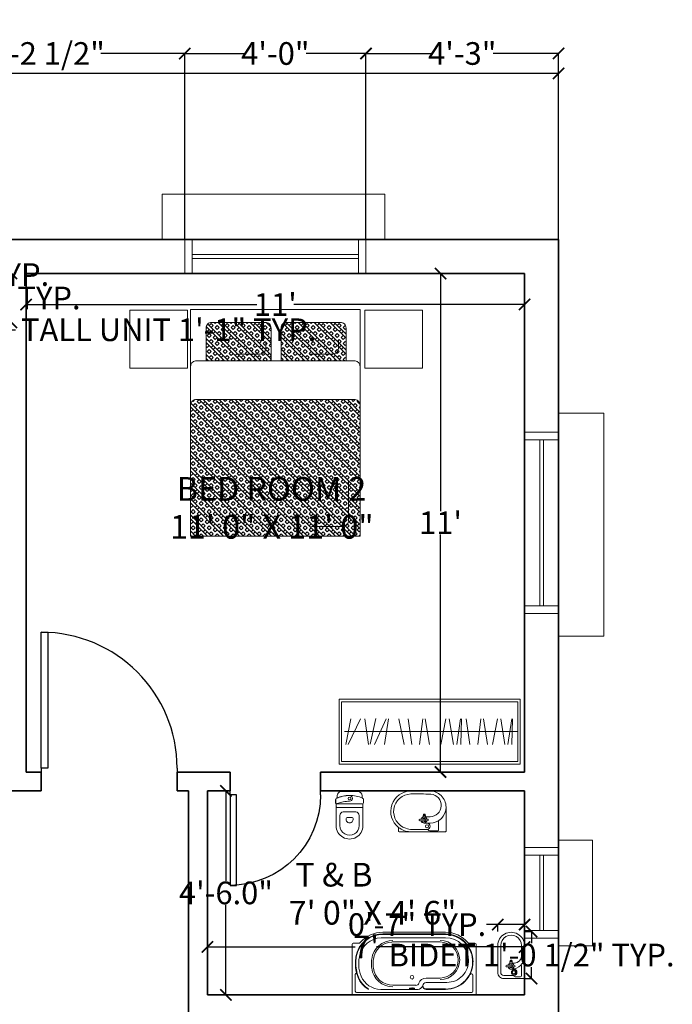
# Model space of a CAD drawing. Units: inches. Extents: x 844 to 2234, y 346 to 1084.
# Tile 46 of 93: x 1287 to 1460, y 823 to 1084. Entities that reach past the tile are written whole.
import ezdxf

# ---------------------------------------------------------------- set-up
doc = ezdxf.new("R2010")
doc.units = ezdxf.units.IN
doc.header["$MEASUREMENT"] = 0
for name, color, linetype, lineweight in [('A-ANNO-DIMS', 2, 'Continuous', 18), ('A-AREA-IDEN', 7, 'Continuous', 18), ('A-FLOR-FIXT', 8, 'Continuous', 18), ('A-WALL', 7, 'Continuous', 35), ('beds', 130, 'Continuous', 18), ('doors', 170, 'Continuous', 25), ('furniture', 8, 'Continuous', 18), ('windows', 1, 'Continuous', 18)]:
    doc.layers.add(name, color=color, linetype=linetype, lineweight=lineweight)
doc.styles.get("Standard").update_dxf_attribs({"font": 'arial.ttf'})
doc.dimstyles.get("Standard").update_dxf_attribs({"dimtxt": 6, "dimasz": 3, "dimexe": 0.18, "dimexo": 0.0625, "dimgap": 0.09, "dimtad": 0, "dimtih": 1, "dimtoh": 1, "dimdec": 1, "dimzin": 0, "dimdsep": 46, "dimlunit": 3, "dimtxsty": 'Standard', "dimblk": 'ARCHTICK', "dimcen": 0.09, "dimadec": 0, "dimazin": 0, "dimtfac": 1, "dimtdec": 1, "dimtofl": 0, "dimtmove": 0, "dimatfit": 3, "dimfxl": 1, "dimtolj": 1, "dimtzin": 0, "dimarcsym": 0})
pattern_1 = [(135, (-1377.70473, -125.71507), (-0.070710678, -0.070710678), []), (135, (-1377.68705, -125.69739), (-0.070710678, -0.070710678), []), (45, (-1377.70473, -125.71507), (-0.070710678, 0.070710678), [-0.025, 0.025]), (45, (-1377.72241, -125.69739), (-0.070710678, 0.070710678), [-0.025, 0.025]), (45, (-1377.74009, -125.67972), (-0.070710678, 0.070710678), [0.025, -0.025]), (45, (-1377.75776, -125.66204), (-0.070710678, 0.070710678), [0.025, -0.025]), (135, (-1377.66938, -125.67972), (-0.070710678, -0.070710678), [0.025, -0.025]), (135, (-1377.6517, -125.66204), (-0.070710678, -0.070710678), [0.025, -0.025])]

# ---------------------------------------------------------------- blocks, each defined once
blk = doc.blocks.new('*U2')
for p, q in [((0, 0), (0, -6)), ((36, 0), (36, -6))]:
    blk.add_line(p, q)
blk.add_lwpolyline([(0, 0), (0, 36), (1.75, 36), (1.75, 0)], close=True)
blk.add_arc((0, 0), 36, 0, 90)
blk = doc.blocks.new('*U4')
for p, q in [((0, 0), (0, -6)), ((24, 0), (24, -6))]:
    blk.add_line(p, q)
blk.add_lwpolyline([(0, 0), (0, 24), (1.75, 24), (1.75, 0)], close=True)
blk.add_arc((0, 0), 24, 0, 90)
blk = doc.blocks.new('MAT-P10')
h = blk.add_hatch()
h.set_pattern_fill('BOX', color=256, scale=0.1, angle=45, style=0)
h.set_pattern_definition(pattern_1)
h.paths.add_polyline_path([(-0.1565, 1.4605), (0.417, 1.4605), (0.417, 1.7513, 0.414214), (0.367, 1.8013), (-0.1065, 1.8013, 0.414214), (-0.1565, 1.7513)])
h.paths.add_polyline_path([(0.5052, 1.4604), (1.0792, 1.4604), (1.0792, 1.7513, 0.414214), (1.0292, 1.8013), (0.5552, 1.8013, 0.414214), (0.5052, 1.7513)])
h = blk.add_hatch()
h.set_pattern_fill('BOX', color=256, scale=0.1, angle=45, style=0)
h.set_pattern_definition(pattern_1)
edge = h.paths.add_edge_path()
edge.add_line((1.2049, -0.085), (1.2049, 1.0625))
edge.add_ellipse((1.1608, 1.0627), major_axis=(0, 0.0568), ratio=0.776379, start_angle=270, end_angle=360)
edge.add_line((1.1608, 1.1195), (-0.251, 1.1195))
edge.add_ellipse((-0.251, 1.0627), major_axis=(0, 0.0568), ratio=0.776379, start_angle=0, end_angle=88.13958)
edge.add_line((-0.2951, 1.0641), (-0.2951, -0.085))
edge.add_line((-0.2951, -0.085), (1.2049, -0.085))
for p, q in [((-0.251, 1.4605), (1.1608, 1.4604)), ((-0.251, 1.1195), (1.1608, 1.1195)), ((1.1017, 0.406), (1.1017, 0.0572)), ((1.0576, 0.0004), (0.7754, 0.0004))]:
    blk.add_line(p, q)
for points in [[(1.2049, -0.085), (-0.2951, -0.085), (-0.2951, 1.9151), (1.2049, 1.915)], [(-0.8301, 1.9091), (-0.3191, 1.9091), (-0.3191, 1.3981), (-0.8301, 1.3981)], [(1.2441, 1.9091), (1.755, 1.9091), (1.755, 1.3981), (1.2441, 1.3981)]]:
    blk.add_lwpolyline(points, close=True)
for points in [[(0.417, 1.4604), (0.417, 1.7513, 0.414214), (0.367, 1.8013), (-0.1065, 1.8013, 0.414214), (-0.1565, 1.7513), (-0.1565, 1.4604)], [(1.0792, 1.4603), (1.0792, 1.7513, 0.414214), (1.0292, 1.8013), (0.5552, 1.8013, 0.414214), (0.5052, 1.7513), (0.5052, 1.4604)], [(0.3702, 1.6242), (0.3702, 1.5715, -0.414214), (0.3202, 1.5215), (0.1113, 1.5215)], [(1.0117, 1.6438), (1.0117, 1.5715, -0.414214), (0.9617, 1.5215), (0.7528, 1.5215)]]:
    blk.add_lwpolyline(points, format="xyb")
at = {"extrusion": (0, 0, -1)}
for centre, start_param, end_param in [((-0.251, 1.4036), 4.712389, 6.283185), ((1.1608, 1.4036), 0, 1.570796), ((-0.251, 1.0627), 4.712389, 6.283185), ((1.1608, 1.0627), 0, 1.570796), ((1.0576, 0.0572), 1.570796, 3.141593), ((1.0576, 0.0572), 1.570796, 3.141593)]:
    blk.add_ellipse(centre, major_axis=(0, 0.0568), ratio=0.776379, start_param=start_param, end_param=end_param, dxfattribs=at)
blk = doc.blocks.new('A$C7A17768A')
for p, q in [((-2.8, 0), (0, 0)), ((-2.8, -1), (-2.8, 0)), ((0, -1), (0, 0)), ((-2.76, -0.04), (-0.04, -0.04)), ((-2.76, -0.96), (-2.76, -0.04)), ((-0.04, -0.96), (-0.04, -0.04)), ((-2.617, -0.3), (-2.694, -0.7)), ((-2.66, -0.7), (-2.466, -0.3)), ((-2.403, -0.3), (-2.342, -0.7)), ((-2.229, -0.296), (-2.317, -0.696)), ((-2.074, -0.3), (-2.25, -0.7)), ((-2.096, -0.7), (-2.033, -0.3)), ((-1.875, -0.3), (-1.796, -0.7)), ((-1.732, -0.3), (-1.675, -0.7)), ((-1.555, -0.7), (-1.507, -0.3)), ((-1.467, -0.3), (-1.403, -0.7)), ((-1.227, -0.7), (-1.151, -0.3)), ((-1.098, -0.3), (-1.034, -0.7)), ((-0.98, -0.7), (-0.921, -0.3)), ((-0.908, -0.3), (-0.919, -0.7)), ((-0.834, -0.3), (-0.777, -0.7)), ((-0.657, -0.7), (-0.61, -0.3)), ((-0.57, -0.3), (-0.505, -0.7)), ((-0.429, -0.7), (-0.353, -0.3)), ((-0.301, -0.3), (-0.237, -0.7)), ((-0.192, -0.7), (-0.133, -0.3)), ((-0.12, -0.3), (-0.131, -0.7)), ((-0.04, -0.5), (-2.716, -0.5)), ((-2.8, -1), (0, -1)), ((-2.76, -0.96), (-0.04, -0.96))]:
    blk.add_line(p, q)
blk = doc.blocks.new('2SABICO')
at = {"color": 0, "linetype": 'ByBlock'}
for p, q in [((0.478, 0.195), (0.089, 0.195)), ((0.478, 0.152), (0.089, 0.152)), ((0, 0.106), (0, 0)), ((0, 0), (0, -0.18)), ((0.043, -0.039), (0.043, 0.106)), ((0.135, 0), (0.135, -0.003)), ((0.168, 0.064), (0.168, -0.015)), ((0.192, 0.064), (0.192, -0.015)), ((0.221, 0.012), (0.222, 0.012)), ((0.223, 0.016), (0.223, -0.016)), ((0.224, 0.017), (0.245, 0.017)), ((0.246, 0.016), (0.246, -0.016)), ((0.25, 0.014), (0.246, 0.014)), ((0.26, 0.01), (0.268, 0.01)), ((0.268, -0.01), (0.268, 0.01)), ((0.268, 0.01), (0.269, 0.009)), ((0.269, -0.009), (0.269, 0.009)), ((0.023, -0.057), (0.023, -0.135)), ((0.135, 0), (0.135, -0.039)), ((0.168, -0.015), (0.192, -0.015)), ((0.168, -0.015), (0.168, -0.046)), ((0.192, -0.015), (0.192, -0.046)), ((0.221, -0.012), (0.222, -0.012)), ((0.224, -0.017), (0.245, -0.017)), ((0.225, -0.017), (0.225, -0.047)), ((0.25, -0.014), (0.246, -0.014)), ((0.26, -0.01), (0.268, -0.01)), ((0.268, -0.01), (0.269, -0.009)), ((0.015, -0.195), (0.478, -0.195)), ((0.038, -0.15), (0.179, -0.15)), ((0.33, -0.152), (0.478, -0.152))]:
    blk.add_line(p, q, dxfattribs=at)
for radius in [0.035, 0.023]:
    blk.add_circle((0.089, -0.039), radius, dxfattribs=at)
for centre, radius, start, end in [((0.089, 0.106), 0.089, 90, 180), ((0.089, 0.106), 0.046, 90, 180), ((0.478, 0), 0.195, 270, 90), ((0.478, 0), 0.152, 270, 90), ((0.18, 0), 0.045, 105.6643, 180), ((0.18, 0), 0.042, 106.8152, 252.6853), ((0.18, 0), 0.0235, 121.1327, 237.8651), ((0.18, 0.064), 0.0121, 0, 180), ((0.18, 0), 0.045, 17.0576, 74.3357), ((0.18, 0), 0.042, 287.3147, 73.1848), ((0.18, 0), 0.0235, 302.1349, 58.8673), ((0.221, 0.013), 0.001, 197.9471, 270), ((0.222, 0.013), 0.001, 270, 0), ((0.224, 0.016), 0.001, 90, 180), ((0.245, 0.016), 0.001, 0, 90), ((0.25, 0), 0.0143, 270, 90), ((0.041, -0.057), 0.018, 99.5941, 180), ((0.038, -0.135), 0.015, 180, 270), ((0.037, -0.033), 0.006, 279.5941, 0), ((0.089, -0.039), 0.046, 180, 360), ((0.326, -0.003), 0.191, 180, 270), ((0.18, -0.046), 0.0125, 180, 0), ((0.179, -0.14), 0.01, 270, 42.9682), ((0.221, -0.013), 0.001, 90, 162.0529), ((0.222, -0.013), 0.001, 0, 90), ((0.224, -0.016), 0.001, 180, 270), ((0.33, -0.047), 0.105, 180, 270), ((0.245, -0.016), 0.001, 270, 0), ((0.015, -0.18), 0.015, 180, 270)]:
    blk.add_arc(centre, radius, start, end, dxfattribs=at)
blk = doc.blocks.new('2SAINCO')
at = {"color": 0, "linetype": 'ByBlock'}
for p, q in [((0.06, 0.181), (0.085, 0.181)), ((0.114, 0.203), (0.165, 0.203)), ((0.496, 0.195), (0.178, 0.195)), ((0.18, -0.188), (0.18, 0.188)), ((0.231, 0.185), (0.231, -0.185)), ((0.234, 0.185), (0.234, -0.185)), ((0, -0.121), (0, 0.121)), ((0.496, 0.14), (0.347, 0.14)), ((0.394, 0.05), (0.407, 0.05)), ((0.496, -0.14), (0.347, -0.14)), ((0.394, -0.05), (0.407, -0.05)), ((0.06, -0.181), (0.085, -0.181)), ((0.114, -0.201), (0.165, -0.201)), ((0.114, -0.203), (0.165, -0.203)), ((0.496, -0.195), (0.178, -0.195))]:
    blk.add_line(p, q, dxfattribs=at)
blk.add_circle((0.1, 0), 0.02, dxfattribs=at)
for centre, radius, start, end in [((0.06, 0.121), 0.06, 90, 180), ((0.517, 0), 0.46, 155.909, 204.091), ((0.085, 0.196), 0.015, 270, 344.534), ((0.114, 0.188), 0.015, 90, 164.534), ((0.165, 0.188), 0.015, 0, 90), ((0.221, 0.185), 0.01, 0, 90), ((0.224, 0.185), 0.01, 0, 90), ((0.496, 0), 0.195, 270, 90), ((0.1, 0), 0.0405, 360, 180), ((0.517, 0), 0.458, 180, 204.67), ((0.66, 0.008), 0.52, 180.891, 201.3823), ((2.295, 0), 2, 177.3546, 182.6454), ((0.347, 0.09), 0.05, 90, 177.3546), ((0.677, 0), 0.3, 172.9459, 187.0541), ((0.394, 0.035), 0.015, 90, 172.9459), ((0.407, 0), 0.05, 270, 90), ((0.496, 0), 0.14, 270, 90), ((0.06, -0.121), 0.06, 180, 270), ((0.347, -0.09), 0.05, 182.6454, 270), ((0.394, -0.035), 0.015, 187.0541, 270), ((0.085, -0.196), 0.015, 15.466, 90), ((0.114, -0.188), 0.015, 195.466, 270), ((0.114, -0.188), 0.013, 195.466, 270), ((0.165, -0.188), 0.013, 270, 30), ((0.165, -0.188), 0.015, 270, 0), ((0.221, -0.185), 0.01, 270, 0), ((0.224, -0.185), 0.01, 270, 0)]:
    blk.add_arc(centre, radius, start, end, dxfattribs=at)
blk = doc.blocks.new('2SABACO')
at = {"color": 0}
for p, q in [((1.341, 0.91), (0.429, 0.91)), ((1.341, 0.885), (0.429, 0.885)), ((1.341, 0.879), (0.429, 0.879)), ((-0.015, 0.735), (-0.015, 0.015)), ((0, 0.75), (0.08, 0.75)), ((1.341, 0.831), (0.407, 0.831)), ((1.263, 0.769), (0.562, 0.769)), ((1.77, 0.75), (1.69, 0.75)), ((1.785, 0.015), (1.785, 0.735)), ((0.03, 0.302), (0.03, 0.053)), ((1.263, 0.245), (1.06, 0.245)), ((1.363, 0.181), (1.06, 0.181)), ((1.74, 0.053), (1.74, 0.286)), ((0, 0), (1.77, 0)), ((0.048, 0.035), (1.722, 0.035)), ((0.401, 0.08), (0.942, 0.08)), ((0.578, 0.139), (0.911, 0.139)), ((1.343, 0.086), (1.06, 0.086)), ((1.343, 0.079), (1.06, 0.079))]:
    blk.add_line(p, q, dxfattribs=at)
blk.add_circle((0.855, 0.256), 0.026, dxfattribs=at)
for centre, radius, start, end in [((0.428, 0.49), 0.395, 98.9726, 181.1954), ((0.428, 0.49), 0.389, 98.9726, 181.2301), ((0.429, 0.48), 0.43, 90, 139.2943), ((0.429, 0.48), 0.405, 90, 98.9726), ((0.429, 0.48), 0.399, 90, 98.9726), ((1.341, 0.48), 0.43, 40.7057, 90), ((1.341, 0.485), 0.401, 359.4627, 90), ((1.341, 0.485), 0.394, 3.5237, 90), ((0, 0.735), 0.015, 90, 180), ((0.08, 0.78), 0.03, 270, 319.2943), ((0.425, 0.49), 0.342, 93.1008, 168.0202), ((0.578, 0.481), 0.311, 90, 172.609), ((0.578, 0.481), 0.288, 93.3767, 172.609), ((1.263, 0.507), 0.285, 270, 90), ((1.263, 0.507), 0.262, 270, 90), ((1.341, 0.495), 0.336, 0, 90), ((1.69, 0.78), 0.03, 220.7057, 270), ((1.77, 0.735), 0.015, 0, 90), ((0.559, 0.454), 0.48, 163.1286, 202.3619), ((0.559, 0.454), 0.528, 177.0415, 202.3619), ((0.559, 0.454), 0.521, 177.0156, 202.3619), ((0.79, 0.454), 0.525, 172.609, 180), ((0.79, 0.454), 0.525, 180, 187.391), ((0.79, 0.454), 0.502, 172.609, 180), ((0.79, 0.454), 0.502, 180, 187.391), ((1.343, 0.477), 0.392, 270, 4.5675), ((1.343, 0.477), 0.398, 270, 0.539), ((1.363, 0.495), 0.314, 270, 2.2815), ((0.042, 0.302), 0.0116, 16.3184, 180.0001), ((0.578, 0.427), 0.311, 187.391, 270), ((0.578, 0.427), 0.288, 187.391, 270), ((1.718, 0.286), 0.0222, 0, 152.9966), ((0.401, 0.389), 0.357, 202.3619, 239.8287), ((0.401, 0.389), 0.351, 202.3619, 239.2093), ((0.401, 0.389), 0.309, 202.3619, 270), ((0.911, 0.183), 0.045, 270, 341.2369), ((1.06, 0.133), 0.112, 90, 161.2369), ((1.06, 0.133), 0.0475, 90, 270), ((0, 0.015), 0.015, 180, 270), ((0.048, 0.053), 0.018, 180, 270), ((0.559, 0.454), 0.48, 250.7818, 251.0555), ((0.821, 0.092), 0.00282, 119.7759, 180), ((0.821, 0.092), 0.00282, 180, 240.2241), ((0.837, 0.064), 0.0347, 103.3326, 119.7759), ((0.835, 0.025), 0.071, 96.5949, 102.1924), ((0.837, 0.12), 0.0347, 240.2241, 256.6674), ((0.847, -0.08), 0.177, 92.7417, 96.5949), ((0.848, 0.02), 0.0808, 95.6065, 103.3326), ((0.848, 0.164), 0.0808, 256.6674, 264.3935), ((0.855, -0.252), 0.349, 90, 92.7417), ((0.855, -0.053), 0.153, 90, 95.6065), ((0.855, 0.237), 0.153, 264.3935, 270), ((0.855, -0.053), 0.153, 84.3935, 90), ((0.855, -0.252), 0.349, 87.2583, 90), ((0.855, 0.237), 0.153, 270, 275.6065), ((0.862, 0.02), 0.0808, 76.6674, 84.3935), ((0.862, 0.164), 0.0808, 275.6065, 283.3326), ((0.863, -0.08), 0.177, 83.4051, 87.2583), ((0.873, 0.064), 0.0347, 60.2241, 76.6674), ((0.873, 0.12), 0.0347, 283.3326, 299.7759), ((0.875, 0.025), 0.071, 77.8076, 83.4051), ((0.889, 0.092), 0.00282, 360, 60.2241), ((0.889, 0.092), 0.00282, 299.7759, 360), ((0.942, 0.145), 0.065, 270, 349.4977), ((1.06, 0.133), 0.054, 180, 270), ((1.722, 0.053), 0.018, 270, 0), ((1.77, 0.015), 0.015, 270, 0)]:
    blk.add_arc(centre, radius, start, end, dxfattribs=at)
blk = doc.blocks.new('2SALACO2')
at = {"color": 0}
for p, q in [((0, 0), (-0.392, 0)), ((0.28, 0), (0, 0)), ((-0.402, -0.01), (-0.402, -0.36)), ((-0.293, -0.026), (-0.293, -0.15)), ((-0.283, -0.016), (-0.166, -0.016)), ((-0.169, -0.128), (-0.085, -0.128)), ((-0.112, -0.035), (-0.133, -0.035)), ((-0.124, -0.035), (0.09, -0.035)), ((0.29, -0.01), (0.29, -0.064)), ((-0.102, -0.219), (-0.169, -0.219)), ((-0.1, -0.161), (-0.131, -0.161)), ((-0.1, -0.186), (-0.131, -0.186)), ((-0.102, -0.217), (-0.102, -0.234)), ((-0.07, -0.216), (-0.101, -0.216)), ((-0.07, -0.235), (-0.101, -0.235)), ((-0.1, -0.161), (-0.1, -0.186)), ((-0.021, -0.161), (-0.1, -0.161)), ((-0.021, -0.186), (-0.1, -0.186)), ((-0.098, -0.214), (-0.098, -0.216)), ((-0.097, -0.239), (-0.098, -0.241)), ((-0.098, -0.241), (-0.098, -0.248)), ((-0.098, -0.241), (-0.073, -0.241)), ((-0.073, -0.248), (-0.098, -0.248)), ((-0.097, -0.235), (-0.097, -0.239)), ((-0.074, -0.239), (-0.097, -0.239)), ((-0.097, -0.248), (-0.097, -0.256)), ((-0.073, -0.256), (-0.097, -0.256)), ((-0.097, -0.256), (-0.094, -0.257)), ((-0.077, -0.257), (-0.094, -0.257)), ((-0.073, -0.256), (-0.077, -0.257)), ((-0.074, -0.235), (-0.074, -0.239)), ((-0.074, -0.239), (-0.073, -0.241)), ((-0.073, -0.214), (-0.073, -0.216)), ((-0.073, -0.241), (-0.073, -0.248)), ((-0.073, -0.248), (-0.073, -0.256)), ((-0.069, -0.217), (-0.069, -0.234))]:
    blk.add_line(p, q, dxfattribs=at)
blk.add_lwpolyline([(-0.402, -0.36, 0.423787), (-0.161, -0.593, 0.423787)], format="xyb", dxfattribs=at)
blk.add_circle((-0.124, -0.081), 0.023, dxfattribs=at)
for centre, radius, start, end in [((-0.392, -0.01), 0.01, 90, 180), ((0.28, -0.01), 0.01, 0, 90), ((-0.169, -0.36), 0.233, 90, 180), ((-0.283, -0.026), 0.01, 90, 180), ((-0.124, -0.081), 0.0462, 90, 270), ((-0.166, -0.046), 0.03, 31.2573, 90), ((-0.133, -0.026), 0.009, 211.2573, 270), ((-0.085, -0.173), 0.042, 16.8152, 162.6853), ((-0.085, -0.173), 0.0458, 15.3964, 90), ((0.09, -0.29), 0.255, 68.9449, 90), ((0.105, -0.295), 0.255, 271.0077, 72.4499), ((0.105, -0.297), 0.297, 271.4871, 51.4524), ((0.105, -0.297), 0.297, 51.4524, 87.1707), ((-0.169, -0.383), 0.164, 90, 265.4963), ((-0.285, -0.15), 0.008, 180, 299.1062), ((-0.131, -0.173), 0.0125, 90, 270), ((-0.085, -0.173), 0.042, 197.3147, 343.1848), ((-0.085, -0.173), 0.0235, 31.1327, 147.8651), ((-0.085, -0.173), 0.0235, 212.1349, 328.8673), ((-0.101, -0.217), 0.001, 90, 180), ((-0.101, -0.234), 0.001, 180, 270), ((-0.085, -0.173), 0.0458, 289.9182, 344.6036), ((-0.07, -0.217), 0.001, 0, 90), ((-0.07, -0.234), 0.001, 270, 0), ((-0.021, -0.173), 0.0121, 270, 90), ((0.021, 4.449), 5, 267.6742, 271.0081), ((-0.017, 4.405), 5, 268.3511, 271.4874)]:
    blk.add_arc(centre, radius, start, end, dxfattribs=at)
blk = doc.blocks.new('_ArchTick')
at = {"color": 0, "linetype": 'ByBlock', "const_width": 0.15}
blk.add_lwpolyline([(-0.5, -0.5), (0.5, 0.5)], dxfattribs=at)
blk = doc.blocks.new('*D29')
at = {"layer": 'A-ANNO-DIMS', "color": 0, "lineweight": -2, "transparency": 16777216}
for p, q in [((1398.36, 1016.31), (1398.36, 953.41)), ((1398.42, 1016.31), (1398.54, 1016.31)), ((1398.36, 884.31), (1398.36, 947.21)), ((1398.42, 884.31), (1398.54, 884.31))]:
    blk.add_line(p, q, dxfattribs=at)
at = {"layer": 'Defpoints', "color": 0, "transparency": 16777216}
for p in [(1398.36, 1016.31), (1398.36, 884.31), (1398.36, 884.31)]:
    blk.add_point(p, dxfattribs=at)
at = {"layer": 'A-ANNO-DIMS', "color": 0, "lineweight": -2, "transparency": 16777216, "xscale": 3, "yscale": 3, "zscale": 3}
for p, rotation in [((1398.36, 1016.31), 90), ((1398.36, 884.31), 270)]:
    blk.add_blockref('_ArchTick', p, dxfattribs=dict(at, rotation=rotation))
at = {"layer": 'A-ANNO-DIMS', "color": 0, "transparency": 16777216, "insert": (1398.36, 950.31), "char_height": 6, "attachment_point": 5}
blk.add_mtext("\\A1;11'", dxfattribs=at)
blk = doc.blocks.new('*D30')
at = {"layer": 'A-ANNO-DIMS', "color": 0, "lineweight": -2, "transparency": 16777216}
for p, q in [((1288.62, 1013.89), (1288.62, 1007.92)), ((1420.62, 1013.89), (1420.62, 1007.92)), ((1288.62, 1008.1), (1349.72, 1008.1)), ((1420.62, 1008.1), (1359.51, 1008.1))]:
    blk.add_line(p, q, dxfattribs=at)
at = {"layer": 'Defpoints', "color": 0, "transparency": 16777216}
for p in [(1288.62, 1013.95), (1420.62, 1013.95), (1420.62, 1008.1)]:
    blk.add_point(p, dxfattribs=at)
at = {"layer": 'A-ANNO-DIMS', "color": 0, "lineweight": -2, "transparency": 16777216, "xscale": 3, "yscale": 3, "zscale": 3, "rotation": 180}
blk.add_blockref('_ArchTick', (1288.62, 1008.1), dxfattribs=at)
at = {"layer": 'A-ANNO-DIMS', "color": 0, "lineweight": -2, "transparency": 16777216, "xscale": 3, "yscale": 3, "zscale": 3}
blk.add_blockref('_ArchTick', (1420.62, 1008.1), dxfattribs=at)
at = {"layer": 'A-ANNO-DIMS', "color": 0, "transparency": 16777216, "insert": (1354.62, 1008.1), "char_height": 6, "attachment_point": 5}
blk.add_mtext("\\A1;11'", dxfattribs=at)
blk = doc.blocks.new('*D43')
at = {"layer": 'A-ANNO-DIMS', "color": 0, "lineweight": -2, "transparency": 16777216}
for p, q in [((1339.68, 879.31), (1341.72, 879.31)), ((1341.54, 879.31), (1341.54, 855.46)), ((1341.54, 825.31), (1341.54, 849.16)), ((1339.68, 825.31), (1341.72, 825.31))]:
    blk.add_line(p, q, dxfattribs=at)
at = {"layer": 'Defpoints', "color": 0, "transparency": 16777216}
for p in [(1339.62, 879.31), (1339.62, 825.31), (1341.54, 825.31)]:
    blk.add_point(p, dxfattribs=at)
at = {"layer": 'A-ANNO-DIMS', "color": 0, "lineweight": -2, "transparency": 16777216, "xscale": 3, "yscale": 3, "zscale": 3}
for p, rotation in [((1341.54, 879.31), 90), ((1341.54, 825.31), 270)]:
    blk.add_blockref('_ArchTick', p, dxfattribs=dict(at, rotation=rotation))
at = {"layer": 'A-ANNO-DIMS', "color": 0, "transparency": 16777216, "insert": (1341.54, 852.31), "char_height": 6, "attachment_point": 5}
blk.add_mtext('\\A1;4\'-6.0"', dxfattribs=at)
blk = doc.blocks.new('*D44')
at = {"layer": 'A-ANNO-DIMS', "color": 0, "lineweight": -2, "transparency": 16777216}
for p, q in [((1336.62, 842.25), (1336.62, 837.81)), ((1420.62, 842.25), (1420.62, 837.81)), ((1336.62, 837.99), (1375.79, 837.99)), ((1420.62, 837.99), (1381.44, 837.99))]:
    blk.add_line(p, q, dxfattribs=at)
at = {"layer": 'Defpoints', "color": 0, "transparency": 16777216}
for p in [(1336.62, 842.31), (1420.62, 842.31), (1336.62, 837.99)]:
    blk.add_point(p, dxfattribs=at)
at = {"layer": 'A-ANNO-DIMS', "color": 0, "lineweight": -2, "transparency": 16777216, "xscale": 3, "yscale": 3, "zscale": 3, "rotation": 180}
blk.add_blockref('_ArchTick', (1336.62, 837.99), dxfattribs=at)
at = {"layer": 'A-ANNO-DIMS', "color": 0, "lineweight": -2, "transparency": 16777216, "xscale": 3, "yscale": 3, "zscale": 3}
blk.add_blockref('_ArchTick', (1420.62, 837.99), dxfattribs=at)
at = {"layer": 'A-ANNO-DIMS', "color": 0, "transparency": 16777216, "insert": (1378.62, 837.99), "char_height": 6, "attachment_point": 5}
blk.add_mtext("\\A1;7'", dxfattribs=at)
blk = doc.blocks.new('*D55')
at = {"layer": 'A-ANNO-DIMS', "color": 0, "lineweight": -2, "transparency": 16777216}
for p, q in [((950.62, 1025.37), (950.62, 1069.43)), ((950.62, 1069.25), (1173.9, 1069.25)), ((1429.62, 1069.25), (1206.34, 1069.25)), ((1429.62, 1025.37), (1429.62, 1069.43))]:
    blk.add_line(p, q, dxfattribs=at)
at = {"layer": 'Defpoints', "color": 0, "transparency": 16777216}
for p in [(1429.62, 1069.25), (950.62, 1025.31), (1429.62, 1025.31)]:
    blk.add_point(p, dxfattribs=at)
at = {"layer": 'A-ANNO-DIMS', "color": 0, "lineweight": -2, "transparency": 16777216, "xscale": 3, "yscale": 3, "zscale": 3, "rotation": 180}
blk.add_blockref('_ArchTick', (950.62, 1069.25), dxfattribs=at)
at = {"layer": 'A-ANNO-DIMS', "color": 0, "lineweight": -2, "transparency": 16777216, "xscale": 3, "yscale": 3, "zscale": 3}
blk.add_blockref('_ArchTick', (1429.62, 1069.25), dxfattribs=at)
at = {"layer": 'A-ANNO-DIMS', "color": 0, "transparency": 16777216, "insert": (1190.12, 1069.25), "char_height": 6, "attachment_point": 5}
blk.add_mtext('\\A1;39\'-11.0"', dxfattribs=at)
blk = doc.blocks.new('WIN-48IN')
for p, q in [((0, 9), (0, 21)), ((0, 21), (59, 21)), ((59, 9), (59, 21)), ((6, 9), (0, 9)), ((54, 9), (6, 9)), ((6, 9), (6, 0)), ((8, 9), (8, 0)), ((52, 0), (52, 9)), ((54, 0), (54, 9)), ((54, 9), (59, 9)), ((8, 5), (52, 5)), ((8, 4), (52, 4)), ((6, 0), (54, 0))]:
    blk.add_line(p, q)
blk = doc.blocks.new('WIN-24IN')
for p, q in [((9, 28), (0, 28)), ((0, 0), (0, 28)), ((9, 26), (9, 28)), ((18, 26), (9, 26)), ((9, 26), (9, 2)), ((18, 24), (9, 24)), ((13, 4), (13, 24)), ((14, 4), (14, 24)), ((18, 2), (18, 26)), ((9, 4), (18, 4)), ((9, 2), (18, 2)), ((9, 2), (9, 0)), ((9, 0), (0, 0))]:
    blk.add_line(p, q)
blk = doc.blocks.new('*D111')
at = {"layer": 'A-ANNO-DIMS', "color": 0, "lineweight": -2, "transparency": 16777216}
for p, q in [((1420.68, 842.06), (1422.66, 842.06)), ((1422.48, 842.06), (1422.48, 839.04)), ((1422.48, 829.64), (1422.48, 832.66)), ((1420.68, 829.64), (1422.66, 829.64))]:
    blk.add_line(p, q, dxfattribs=at)
at = {"layer": 'Defpoints', "color": 0, "transparency": 16777216}
for p in [(1420.62, 842.06), (1422.48, 842.06), (1420.62, 829.64)]:
    blk.add_point(p, dxfattribs=at)
at = {"layer": 'A-ANNO-DIMS', "color": 0, "lineweight": -2, "transparency": 16777216, "xscale": 3, "yscale": 3, "zscale": 3}
for p, rotation in [((1422.48, 842.06), 90), ((1422.48, 829.64), 270)]:
    blk.add_blockref('_ArchTick', p, dxfattribs=dict(at, rotation=rotation))
at = {"layer": 'A-ANNO-DIMS', "color": 0, "transparency": 16777216, "insert": (1422.48, 835.85), "char_height": 6, "attachment_point": 5}
blk.add_mtext('\\A1;BIDET 1\'-0 1/2" TYP.', dxfattribs=at)
blk = doc.blocks.new('*D112')
at = {"layer": 'A-ANNO-DIMS', "color": 0, "lineweight": -2, "transparency": 16777216}
for p, q in [((1413.51, 843.92), (1410.51, 843.92)), ((1413.51, 842.12), (1413.51, 844.1)), ((1420.62, 843.92), (1413.51, 843.92)), ((1420.62, 842.12), (1420.62, 844.1))]:
    blk.add_line(p, q, dxfattribs=at)
at = {"layer": 'Defpoints', "color": 0, "transparency": 16777216}
for p in [(1413.51, 843.92), (1413.51, 842.06), (1420.62, 842.06)]:
    blk.add_point(p, dxfattribs=at)
at = {"layer": 'A-ANNO-DIMS', "color": 0, "lineweight": -2, "transparency": 16777216, "xscale": 3, "yscale": 3, "zscale": 3, "rotation": 180}
blk.add_blockref('_ArchTick', (1413.51, 843.92), dxfattribs=at)
at = {"layer": 'A-ANNO-DIMS', "color": 0, "lineweight": -2, "transparency": 16777216, "xscale": 3, "yscale": 3, "zscale": 3}
blk.add_blockref('_ArchTick', (1420.62, 843.92), dxfattribs=at)
at = {"layer": 'A-ANNO-DIMS', "color": 0, "transparency": 16777216, "insert": (1392.14, 843.92), "char_height": 6, "attachment_point": 5}
blk.add_mtext('\\A1;0\'-7" TYP.', dxfattribs=at)
blk = doc.blocks.new('*D125')
at = {"layer": 'A-ANNO-DIMS', "color": 0, "lineweight": -2, "transparency": 16777216}
for p, q in [((1269.83, 1003.29), (1269.83, 1001.23)), ((1269.83, 1001.41), (1282.79, 1001.41)), ((1282.79, 1003.29), (1282.79, 1001.23)), ((1282.79, 1001.41), (1285.79, 1001.41))]:
    blk.add_line(p, q, dxfattribs=at)
at = {"layer": 'Defpoints', "color": 0, "transparency": 16777216}
for p in [(1269.83, 1003.35), (1282.79, 1003.35), (1282.79, 1001.41)]:
    blk.add_point(p, dxfattribs=at)
at = {"layer": 'A-ANNO-DIMS', "color": 0, "lineweight": -2, "transparency": 16777216, "xscale": 3, "yscale": 3, "zscale": 3, "rotation": 180}
blk.add_blockref('_ArchTick', (1269.83, 1001.41), dxfattribs=at)
at = {"layer": 'A-ANNO-DIMS', "color": 0, "lineweight": -2, "transparency": 16777216, "xscale": 3, "yscale": 3, "zscale": 3}
blk.add_blockref('_ArchTick', (1282.79, 1001.41), dxfattribs=at)
at = {"layer": 'A-ANNO-DIMS', "color": 0, "transparency": 16777216, "insert": (1326.36, 1001.41), "char_height": 6, "attachment_point": 5}
blk.add_mtext('\\A1;TALL UNIT 1\'-1" TYP.', dxfattribs=at)
blk = doc.blocks.new('*D126')
at = {"layer": 'A-ANNO-DIMS', "color": 0, "lineweight": -2, "transparency": 16777216}
for p, q in [((1282.85, 1016.31), (1284.91, 1016.31)), ((1284.73, 1016.31), (1284.73, 1012.93)), ((1284.73, 1003.35), (1284.73, 1006.73)), ((1282.85, 1003.35), (1284.91, 1003.35))]:
    blk.add_line(p, q, dxfattribs=at)
at = {"layer": 'Defpoints', "color": 0, "transparency": 16777216}
for p in [(1282.79, 1016.31), (1284.73, 1016.31), (1282.79, 1003.35)]:
    blk.add_point(p, dxfattribs=at)
at = {"layer": 'A-ANNO-DIMS', "color": 0, "lineweight": -2, "transparency": 16777216, "xscale": 3, "yscale": 3, "zscale": 3}
for p, rotation in [((1284.73, 1016.31), 90), ((1284.73, 1003.35), 270)]:
    blk.add_blockref('_ArchTick', p, dxfattribs=dict(at, rotation=rotation))
at = {"layer": 'A-ANNO-DIMS', "color": 0, "transparency": 16777216, "insert": (1284.73, 1009.83), "char_height": 6, "attachment_point": 5}
blk.add_mtext('\\A1;1\'-1" TYP.', dxfattribs=at)
blk = doc.blocks.new('*D133')
at = {"layer": 'A-ANNO-DIMS', "color": 0, "lineweight": -2, "transparency": 16777216}
for p, q in [((1208.76, 1014.21), (1208.76, 1016.21)), ((1208.76, 1016.03), (1221.29, 1016.03)), ((1221.29, 1014.21), (1221.29, 1016.21)), ((1221.29, 1016.03), (1224.29, 1016.03))]:
    blk.add_line(p, q, dxfattribs=at)
at = {"layer": 'Defpoints', "color": 0, "transparency": 16777216}
for p in [(1208.76, 1014.15), (1221.29, 1016.03), (1221.29, 1014.15)]:
    blk.add_point(p, dxfattribs=at)
at = {"layer": 'A-ANNO-DIMS', "color": 0, "lineweight": -2, "transparency": 16777216, "xscale": 3, "yscale": 3, "zscale": 3, "rotation": 180}
blk.add_blockref('_ArchTick', (1208.76, 1016.03), dxfattribs=at)
at = {"layer": 'A-ANNO-DIMS', "color": 0, "lineweight": -2, "transparency": 16777216, "xscale": 3, "yscale": 3, "zscale": 3}
blk.add_blockref('_ArchTick', (1221.29, 1016.03), dxfattribs=at)
at = {"layer": 'A-ANNO-DIMS', "color": 0, "transparency": 16777216, "insert": (1259.74, 1016.03), "char_height": 6, "attachment_point": 5}
blk.add_mtext('\\A1;HOB 1\'-0 1/2" TYP.', dxfattribs=at)
blk = doc.blocks.new('*D156')
at = {"layer": 'A-ANNO-DIMS', "color": 0, "lineweight": -2, "transparency": 16777216}
for p, q in [((1256.12, 1025.37), (1256.12, 1074.74)), ((1256.12, 1074.56), (1278.29, 1074.56)), ((1330.62, 1074.56), (1308.44, 1074.56)), ((1330.62, 1025.37), (1330.62, 1074.74))]:
    blk.add_line(p, q, dxfattribs=at)
at = {"layer": 'Defpoints', "color": 0, "transparency": 16777216}
for p in [(1330.62, 1074.56), (1256.12, 1025.31), (1330.62, 1025.31)]:
    blk.add_point(p, dxfattribs=at)
at = {"layer": 'A-ANNO-DIMS', "color": 0, "lineweight": -2, "transparency": 16777216, "xscale": 3, "yscale": 3, "zscale": 3, "rotation": 180}
blk.add_blockref('_ArchTick', (1256.12, 1074.56), dxfattribs=at)
at = {"layer": 'A-ANNO-DIMS', "color": 0, "lineweight": -2, "transparency": 16777216, "xscale": 3, "yscale": 3, "zscale": 3}
blk.add_blockref('_ArchTick', (1330.62, 1074.56), dxfattribs=at)
at = {"layer": 'A-ANNO-DIMS', "color": 0, "transparency": 16777216, "insert": (1293.37, 1074.56), "char_height": 6, "attachment_point": 5}
blk.add_mtext('\\A1;6\'-2 1/2"', dxfattribs=at)
blk = doc.blocks.new('*D157')
at = {"layer": 'A-ANNO-DIMS', "color": 0, "lineweight": -2, "transparency": 16777216}
for p, q in [((1330.62, 1025.37), (1330.62, 1074.74)), ((1330.62, 1074.56), (1346.43, 1074.56)), ((1378.62, 1074.56), (1362.8, 1074.56)), ((1378.62, 1025.37), (1378.62, 1074.74))]:
    blk.add_line(p, q, dxfattribs=at)
at = {"layer": 'Defpoints', "color": 0, "transparency": 16777216}
for p in [(1378.62, 1074.56), (1330.62, 1025.31), (1378.62, 1025.31)]:
    blk.add_point(p, dxfattribs=at)
at = {"layer": 'A-ANNO-DIMS', "color": 0, "lineweight": -2, "transparency": 16777216, "xscale": 3, "yscale": 3, "zscale": 3, "rotation": 180}
blk.add_blockref('_ArchTick', (1330.62, 1074.56), dxfattribs=at)
at = {"layer": 'A-ANNO-DIMS', "color": 0, "lineweight": -2, "transparency": 16777216, "xscale": 3, "yscale": 3, "zscale": 3}
blk.add_blockref('_ArchTick', (1378.62, 1074.56), dxfattribs=at)
at = {"layer": 'A-ANNO-DIMS', "color": 0, "transparency": 16777216, "insert": (1354.62, 1074.56), "char_height": 6, "attachment_point": 5}
blk.add_mtext('\\A1;4\'-0"', dxfattribs=at)
blk = doc.blocks.new('*D158')
at = {"layer": 'A-ANNO-DIMS', "color": 0, "lineweight": -2, "transparency": 16777216}
for p, q in [((1378.62, 1025.37), (1378.62, 1074.74)), ((1378.62, 1074.56), (1395.93, 1074.56)), ((1429.62, 1074.56), (1412.3, 1074.56)), ((1429.62, 1025.37), (1429.62, 1074.74))]:
    blk.add_line(p, q, dxfattribs=at)
at = {"layer": 'Defpoints', "color": 0, "transparency": 16777216}
for p in [(1429.62, 1074.56), (1378.62, 1025.31), (1429.62, 1025.31)]:
    blk.add_point(p, dxfattribs=at)
at = {"layer": 'A-ANNO-DIMS', "color": 0, "lineweight": -2, "transparency": 16777216, "xscale": 3, "yscale": 3, "zscale": 3, "rotation": 180}
blk.add_blockref('_ArchTick', (1378.62, 1074.56), dxfattribs=at)
at = {"layer": 'A-ANNO-DIMS', "color": 0, "lineweight": -2, "transparency": 16777216, "xscale": 3, "yscale": 3, "zscale": 3}
blk.add_blockref('_ArchTick', (1429.62, 1074.56), dxfattribs=at)
at = {"layer": 'A-ANNO-DIMS', "color": 0, "transparency": 16777216, "insert": (1404.12, 1074.56), "char_height": 6, "attachment_point": 5}
blk.add_mtext('\\A1;4\'-3"', dxfattribs=at)

msp = doc.modelspace()

# ---------------------------------------------------------------- linework, layer by layer
at = {"layer": 'A-WALL'}
for p, q in [((950.62, 1025.31), (1429.62, 1025.31)), ((1429.62, 1025.31), (1429.62, 430.31)), ((1288.62, 1016.31), (1288.62, 884.31)), ((1288.62, 1016.31), (1420.62, 1016.31)), ((1420.62, 1016.31), (1420.62, 884.31)), ((1288.62, 884.31), (1292.62, 884.31)), ((1292.62, 884.31), (1292.62, 879.31)), ((1328.62, 884.31), (1328.62, 879.31)), ((1328.62, 884.31), (1342.62, 884.31)), ((1342.62, 879.31), (1342.62, 884.31)), ((1366.62, 879.31), (1366.62, 884.31)), ((1366.62, 884.31), (1420.62, 884.31)), ((1240.62, 879.31), (1292.62, 879.31)), ((1328.62, 879.31), (1331.62, 879.31)), ((1331.62, 879.31), (1331.62, 790.31)), ((1336.62, 879.31), (1336.62, 825.31)), ((1336.62, 879.31), (1342.62, 879.31)), ((1366.62, 879.31), (1420.62, 879.31)), ((1420.62, 879.31), (1420.62, 825.31)), ((1420.62, 825.31), (1336.62, 825.31))]:
    msp.add_line(p, q, dxfattribs=at)

# ---------------------------------------------------------------- block references
at = {"layer": 'A-FLOR-FIXT', "xscale": 18.21101258924898, "yscale": 18.21101258924898, "zscale": 18.21101258924898}
for name, p, rotation in [('2SAINCO', (1374.28, 879.15), 270), ('2SALACO2', (1392.5, 868.48), 180), ('2SABICO', (1417.06, 829.64), 89.99999999999999)]:
    msp.add_blockref(name, p, dxfattribs=dict(at, rotation=rotation))
msp.add_blockref('2SABACO', (1375.25, 825.31), dxfattribs=at)
at = {"layer": 'beds', "xscale": 29.99962925113936, "yscale": 29.99962925113936, "zscale": 29.99962925113936}
msp.add_blockref('MAT-P10', (1340.97, 949.34), dxfattribs=at)
at = {"layer": 'doors'}
msp.add_blockref('*U2', (1292.62, 885.31), dxfattribs=at)
at = {"layer": 'doors', "xscale": -1, "rotation": 180}
msp.add_blockref('*U4', (1342.62, 878.31), dxfattribs=at)
at = {"layer": 'furniture', "xscale": 17.14285714285603, "yscale": 17.14285714285603, "zscale": 17.14285714285603}
msp.add_blockref('A$C7A17768A', (1419.48, 903.58), dxfattribs=at)
at = {"layer": 'windows'}
msp.add_blockref('WIN-48IN', (1324.62, 1016.31), dxfattribs=at)
at = {"layer": 'windows', "extrusion": (0, 0, -1), "zscale": -1, "rotation": 90.00000000000178}
msp.add_blockref('WIN-48IN', (-1420.62, 920.31), dxfattribs=at)
at = {"layer": 'windows', "rotation": 180}
msp.add_blockref('WIN-24IN', (1438.62, 866.31), dxfattribs=at)

# ---------------------------------------------------------------- texts
at = {"layer": 'A-AREA-IDEN'}
for s, height, p in [('BED ROOM 2', 6.269, (1328.52, 956.15)), (' 11\' 0" X 11\' 0"', 6.2688, (1324.82, 946.08)), ('T & B', 6.269, (1359.95, 853.99)), (' 7\' 0" X 4\' 6"', 6.2688, (1356.25, 843.92))]:
    msp.add_text(s, height=height, dxfattribs=at).set_placement(p)

# ---------------------------------------------------------------- dimensions: what is measured, and where the dimension line sits
at = {"layer": 'A-ANNO-DIMS'}
for base, p1, p2, override, picture, middle in [((1330.62, 1074.56), (1256.12, 1025.31), (1330.62, 1025.31), {"dimdec": 1, "dimlfac": 1, "dimrnd": 0, "dimzin": 1, "dimdsep": 46, "dimlunit": 4, "dimfrac": 2}, '*D156', (1293.37, 1074.56)), ((1378.62, 1074.56), (1330.62, 1025.31), (1378.62, 1025.31), {"dimdec": 1, "dimlfac": 1, "dimrnd": 0, "dimzin": 1, "dimdsep": 46, "dimlunit": 4, "dimfrac": 2}, '*D157', (1354.62, 1074.56)), ((1429.62, 1074.56), (1378.62, 1025.31), (1429.62, 1025.31), {"dimdec": 1, "dimlfac": 1, "dimrnd": 0, "dimzin": 1, "dimdsep": 46, "dimlunit": 4, "dimfrac": 2}, '*D158', (1404.12, 1074.56)), ((1429.62, 1069.25), (950.62, 1025.31), (1429.62, 1025.31), {"dimclrd": 0, "dimclre": 0, "dimclrt": 0}, '*D55', (1190.12, 1069.25)), ((1420.62, 1008.1), (1288.62, 1013.95), (1420.62, 1013.95), {"dimclrd": 0, "dimclre": 0, "dimclrt": 0}, '*D30', (1354.62, 1008.1)), ((1336.62, 837.99), (1420.62, 842.31), (1336.62, 842.31), {"dimclrd": 0, "dimclre": 0, "dimclrt": 0}, '*D44', (1378.62, 837.99))]:
    dim = msp.add_linear_dim(base=base, p1=p1, p2=p2, dimstyle='Standard', override=override, dxfattribs=at)
    dim.commit()
    dim.dimension.update_dxf_attribs({"geometry": picture, "text_midpoint": middle})
for base, p1, p2, text, picture, middle in [((1221.29, 1016.03), (1208.76, 1014.15), (1221.29, 1014.15), 'HOB <> TYP.', '*D133', (1259.74, 1016.03)), ((1282.79, 1001.41), (1269.83, 1003.35), (1282.79, 1003.35), 'TALL UNIT <> TYP.', '*D125', (1326.36, 1001.41))]:
    dim = msp.add_linear_dim(base=base, p1=p1, p2=p2, text=text, dimstyle='Standard', override={"dimdec": 1, "dimlfac": 1, "dimrnd": 0, "dimzin": 1, "dimdsep": 46, "dimlunit": 4, "dimfrac": 2}, dxfattribs=at)
    dim.commit()
    dim.dimension.update_dxf_attribs({"geometry": picture, "text_midpoint": middle})
for base, p1, p2, angle, text, picture, middle in [((1284.73, 1016.31), (1282.79, 1003.35), (1282.79, 1016.31), 90, '<> TYP.', '*D126', (1284.73, 1009.83)), ((1413.51, 843.92), (1420.62, 842.06), (1413.51, 842.06), 180, '<> TYP.', '*D112', (1392.14, 843.92)), ((1422.48, 842.06), (1420.62, 829.64), (1420.62, 842.06), 90, 'BIDET <> TYP.', '*D111', (1422.48, 835.85))]:
    dim = msp.add_linear_dim(base=base, p1=p1, p2=p2, angle=angle, text=text, dimstyle='Standard', override={"dimdec": 1, "dimlfac": 1, "dimrnd": 0, "dimzin": 1, "dimdsep": 46, "dimlunit": 4, "dimfrac": 2}, dxfattribs=at)
    dim.commit()
    dim.dimension.update_dxf_attribs({"geometry": picture, "text_midpoint": middle})
for base, p1, p2, picture, middle in [((1398.36, 884.31), (1398.36, 1016.31), (1398.36, 884.31), '*D29', (1398.36, 950.31)), ((1341.54, 825.31), (1339.62, 879.31), (1339.62, 825.31), '*D43', (1341.54, 852.31))]:
    dim = msp.add_linear_dim(base=base, p1=p1, p2=p2, angle=90, dimstyle='Standard', override={"dimclrd": 0, "dimclre": 0, "dimclrt": 0}, dxfattribs=at)
    dim.commit()
    dim.dimension.update_dxf_attribs({"geometry": picture, "text_midpoint": middle})

doc.saveas('drawing.dxf')
